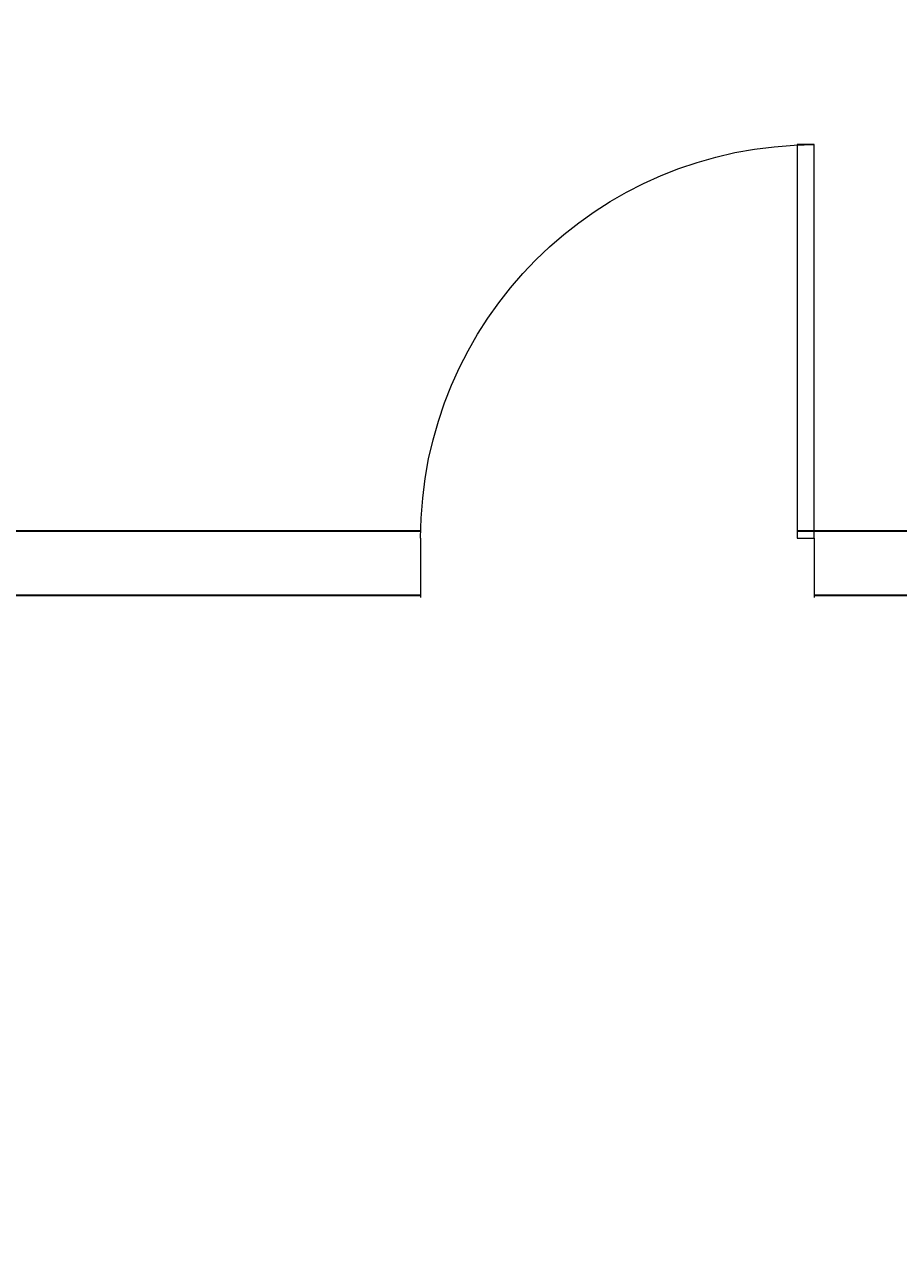
# Model space of a CAD drawing. Units: millimetres. Extents: x 27017497 to 27018854, y 7058029 to 7059154.
# Tile 42 of 91: x 27017689 to 27017750, y 7058386 to 7058472. Entities that reach past the tile are written whole.
import ezdxf

# ---------------------------------------------------------------- set-up
doc = ezdxf.new("R2010")
doc.units = ezdxf.units.MM
for name, color, linetype, lineweight in [('A-ANNO-DIMS', 2, 'Continuous', 18), ('A-DOOR', 4, 'Continuous', 20), ('A-WALL', 7, 'Continuous', 35)]:
    doc.layers.add(name, color=color, linetype=linetype, lineweight=lineweight)
doc.styles.get("Standard").update_dxf_attribs({"font": 'arial.ttf'})
doc.dimstyles.get("Standard").update_dxf_attribs({"dimtxt": 0.18, "dimasz": 0.18, "dimexe": 0.18, "dimexo": 0.0625, "dimgap": 0.09, "dimtad": 0, "dimtih": 1, "dimtoh": 1, "dimdec": 4, "dimzin": 0, "dimdsep": 46, "dimtxsty": 'Standard', "dimcen": 0.09, "dimadec": 0, "dimazin": 0, "dimtfac": 1, "dimtdec": 4, "dimtofl": 0, "dimtmove": 0, "dimatfit": 3, "dimfxl": 1, "dimtolj": 1, "dimtzin": 0, "dimarcsym": 0})

# ---------------------------------------------------------------- blocks, each defined once
blk = doc.blocks.new('*U2')
for p, q in [((0, 0), (0, -6)), ((40, 0), (40, -6))]:
    blk.add_line(p, q)
blk.add_lwpolyline([(0, 0), (0, 40), (1.75, 40), (1.75, 0)], close=True)
blk.add_arc((0, 0), 40, 0, 90)
blk = doc.blocks.new('*D48')
at = {"layer": 'A-ANNO-DIMS', "color": 0, "lineweight": -2, "transparency": 16777216}
for p, q in [((27018463.498, 7058622.912), (27017497.536, 7058622.912)), ((27017497.716, 7058622.732), (27017497.716, 7058357.753)), ((27017497.716, 7058092.41), (27017497.716, 7058357.389)), ((27018555.129, 7058092.23), (27017497.536, 7058092.23))]:
    blk.add_line(p, q, dxfattribs=at)
at = {"layer": 'A-ANNO-DIMS', "color": 0, "transparency": 16777216}
for points in [[(27017497.686, 7058622.732), (27017497.746, 7058622.732), (27017497.716, 7058622.912)], [(27017497.686, 7058092.41), (27017497.746, 7058092.41), (27017497.716, 7058092.23)]]:
    blk.add_solid(points, dxfattribs=at)
at = {"layer": 'Defpoints', "color": 0, "transparency": 16777216}
for p in [(27018463.561, 7058622.912), (27017497.716, 7058092.23), (27018555.192, 7058092.23)]:
    blk.add_point(p, dxfattribs=at)
at = {"layer": 'A-ANNO-DIMS', "color": 0, "transparency": 16777216, "insert": (27017497.716, 7058357.571), "char_height": 0.18, "attachment_point": 5}
blk.add_mtext('\\A1;530.7', dxfattribs=at)

msp = doc.modelspace()

# ---------------------------------------------------------------- linework, layer by layer
at = {"layer": 'A-WALL'}
for p, q in [((27017622.666, 7058436.912), (27017716.811, 7058436.912)), ((27017743.085, 7058436.912), (27017754.666, 7058436.912)), ((27017641.166, 7058432.412), (27017716.805, 7058432.412)), ((27017744.287, 7058432.412), (27017759.166, 7058432.412))]:
    msp.add_line(p, q, dxfattribs=at)

# ---------------------------------------------------------------- block references
at = {"layer": 'A-DOOR', "xscale": -0.6870473523349573, "yscale": 0.6870473523349573, "zscale": 0.6870473523349573}
msp.add_blockref('*U2', (27017744.287, 7058436.382), dxfattribs=at)

# ---------------------------------------------------------------- dimensions: what is measured, and where the dimension line sits
at = {"layer": 'A-ANNO-DIMS'}
dim = msp.add_linear_dim(base=(27017497.716, 7058092.23), p1=(27018463.561, 7058622.912), p2=(27018555.192, 7058092.23), angle=90, dimstyle='Standard', override={"dimdec": 1, "dimlfac": 1, "dimrnd": 0, "dimzin": 0, "dimdsep": 46, "dimlunit": 2}, dxfattribs=at)
dim.commit()
dim.dimension.update_dxf_attribs({"geometry": '*D48', "text_midpoint": (27017497.716, 7058357.571)})

doc.saveas('drawing.dxf')
